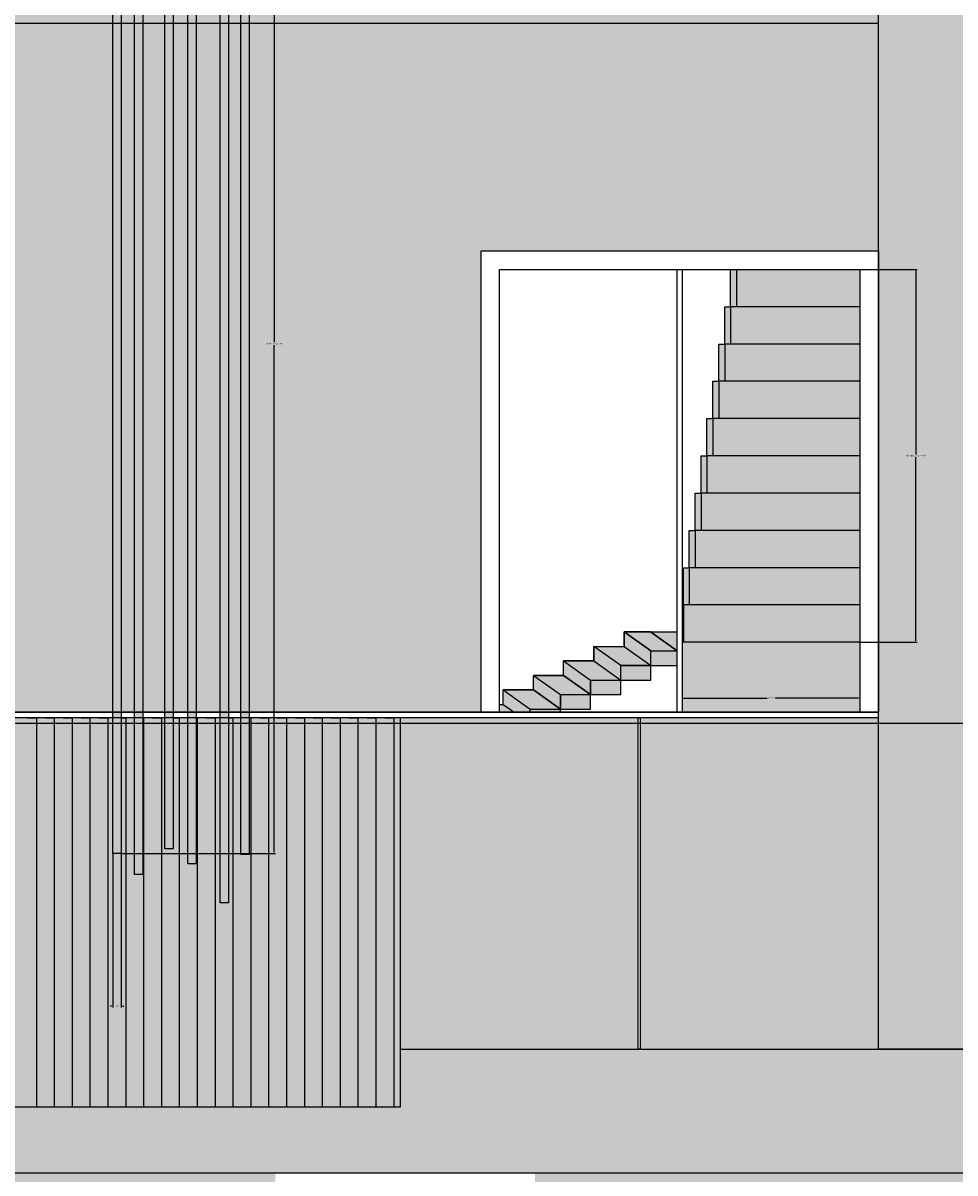
# Model space of a CAD drawing. Units: feet. Extents: x 2193 to 3502, y 890 to 1601.
# Tile 5 of 17: x 2587 to 2710, y 1073 to 1225. Entities that reach past the tile are written whole.
import ezdxf

# ---------------------------------------------------------------- set-up
doc = ezdxf.new("R2010")
doc.units = ezdxf.units.FT
for name, color, linetype, lineweight in [('A-ANNO-DIMS', 2, 'Continuous', 18), ('A-ELEV', 7, 'Continuous', 25), ('A-ELEV-PATT', 8, 'Continuous', 13)]:
    doc.layers.add(name, color=color, linetype=linetype, lineweight=lineweight)
doc.styles.get("Standard").update_dxf_attribs({"font": 'arial.ttf'})
doc.dimstyles.get("Standard").update_dxf_attribs({"dimtxt": 0.18, "dimasz": 0.18, "dimexe": 0.18, "dimexo": 0.0625, "dimgap": 0.09, "dimtad": 0, "dimtih": 1, "dimtoh": 1, "dimdec": 0, "dimzin": 0, "dimdsep": 46, "dimlunit": 3, "dimtxsty": 'Standard', "dimcen": 0.09, "dimadec": 0, "dimazin": 0, "dimtfac": 1, "dimtdec": 0, "dimtofl": 0, "dimtmove": 0, "dimatfit": 3, "dimfxl": 1, "dimtolj": 1, "dimtzin": 0, "dimarcsym": 0})

# ---------------------------------------------------------------- blocks, each defined once
blk = doc.blocks.new('STAIR-RAIL-A')
for p, q in [((6.38, 44.29), (6.38, 49.22)), ((5.61, 39.37), (5.61, 44.29)), ((5.61, 44.29), (6.38, 44.29)), ((23.45, 44.29), (6.38, 44.29)), ((6.38, 44.29), (6.38, 39.37)), ((4.83, 34.45), (4.83, 39.37)), ((4.83, 39.37), (5.61, 39.37)), ((23.45, 39.37), (5.61, 39.37)), ((5.61, 39.37), (5.61, 34.45)), ((4.05, 29.53), (4.05, 34.45)), ((4.05, 34.45), (4.83, 34.45)), ((23.45, 34.45), (4.83, 34.45)), ((4.83, 34.45), (4.83, 29.53)), ((3.27, 24.61), (3.27, 29.53)), ((3.27, 29.53), (4.05, 29.53)), ((23.45, 29.53), (4.05, 29.53)), ((4.05, 29.53), (4.05, 24.61)), ((2.49, 19.69), (2.49, 24.61)), ((2.49, 24.61), (3.27, 24.61)), ((23.45, 24.61), (3.27, 24.61)), ((3.27, 24.61), (3.27, 19.69)), ((1.71, 14.77), (1.71, 19.69)), ((1.71, 19.69), (2.49, 19.69)), ((23.45, 19.69), (2.49, 19.69)), ((2.49, 19.69), (2.49, 14.77)), ((0.93, 9.84), (0.93, 14.77)), ((0.93, 14.77), (1.71, 14.77)), ((23.45, 14.77), (1.71, 14.77)), ((1.71, 14.77), (1.71, 9.84)), ((0.16, 4.92), (0.16, 9.84)), ((0.16, 9.84), (0.93, 9.84)), ((23.45, 9.84), (0.93, 9.84)), ((0.93, 9.84), (0.93, 4.92)), ((23.45, 4.92), (0, 4.92)), ((23.45, 4.92), (0, 4.92)), ((0.16, 4.92), (0.16, 0)), ((23.45, 0), (0, 0)), ((23.45, 0), (0, 0))]:
    blk.add_line(p, q)
for points in [[(23.45, 44.29), (6.38, 44.29), (6.38, 49.22)], [(23.45, 39.37), (5.61, 39.37), (5.61, 44.29), (6.38, 44.29), (6.38, 39.37)], [(23.45, 34.45), (4.83, 34.45), (4.83, 39.37), (5.61, 39.37), (5.61, 34.45)], [(23.45, 29.53), (4.05, 29.53), (4.05, 34.45), (4.83, 34.45), (4.83, 29.53)], [(23.45, 24.61), (3.27, 24.61), (3.27, 29.53), (4.05, 29.53), (4.05, 24.61)], [(23.45, 19.69), (2.49, 19.69), (2.49, 24.61), (3.27, 24.61), (3.27, 19.69)], [(23.45, 14.77), (1.71, 14.77), (1.71, 19.69), (2.49, 19.69), (2.49, 14.77)], [(23.45, 9.84), (0.93, 9.84), (0.93, 14.77), (1.71, 14.77), (1.71, 9.84)], [(0.16, 0), (0.16, 4.92), (0.16, 9.84), (0.93, 9.84), (0.93, 4.92)]]:
    blk.add_lwpolyline(points)
blk = doc.blocks.new('METAL-FIN')
blk.add_lwpolyline([(0, 134.59), (1.1, 134.59), (1.1, 0), (0, 0)], close=True)
blk.add_lwpolyline([(0, 134.59), (1.1, 134.59), (1.1, 0), (0, 0)], close=True)
blk = doc.blocks.new('*D5')
at = {"layer": 'A-ANNO-DIMS', "color": 0, "lineweight": -2, "transparency": 16777216}
for p, q in [((2599.75, 1249.83), (2620.06, 1249.83)), ((2619.88, 1249.65), (2619.88, 1182.71)), ((2619.88, 1115.41), (2619.88, 1182.35)), ((2599.75, 1115.23), (2620.06, 1115.23))]:
    blk.add_line(p, q, dxfattribs=at)
at = {"layer": 'A-ANNO-DIMS', "color": 0, "transparency": 16777216}
for points in [[(2619.85, 1249.65), (2619.91, 1249.65), (2619.88, 1249.83)], [(2619.85, 1115.41), (2619.91, 1115.41), (2619.88, 1115.23)]]:
    blk.add_solid(points, dxfattribs=at)
at = {"layer": 'Defpoints', "color": 0, "transparency": 16777216}
for p in [(2599.69, 1249.83), (2619.88, 1249.83), (2599.69, 1115.23)]:
    blk.add_point(p, dxfattribs=at)
at = {"layer": 'A-ANNO-DIMS', "color": 0, "transparency": 16777216, "insert": (2619.88, 1182.53), "char_height": 0.18, "attachment_point": 5}
blk.add_mtext('\\A1;METAL FIN 135 TYP.', dxfattribs=at)
blk = doc.blocks.new('*D6')
at = {"layer": 'A-ANNO-DIMS', "color": 0, "lineweight": -2, "transparency": 16777216}
for p, q in [((2598.59, 1115.17), (2598.59, 1094.86)), ((2599.69, 1115.17), (2599.69, 1094.86)), ((2598.41, 1095.04), (2598.23, 1095.04)), ((2599.87, 1095.04), (2600.05, 1095.04))]:
    blk.add_line(p, q, dxfattribs=at)
at = {"layer": 'A-ANNO-DIMS', "color": 0, "transparency": 16777216}
for points in [[(2598.41, 1095.07), (2598.41, 1095.01), (2598.59, 1095.04)], [(2599.87, 1095.07), (2599.87, 1095.01), (2599.69, 1095.04)]]:
    blk.add_solid(points, dxfattribs=at)
at = {"layer": 'Defpoints', "color": 0, "transparency": 16777216}
for p in [(2598.59, 1115.23), (2599.69, 1115.23), (2599.69, 1095.04)]:
    blk.add_point(p, dxfattribs=at)
at = {"layer": 'A-ANNO-DIMS', "color": 0, "transparency": 16777216, "insert": (2599.14, 1095.04), "char_height": 0.18, "attachment_point": 5}
blk.add_mtext('\\A1;1 TYP.', dxfattribs=at)
blk = doc.blocks.new('*D7')
at = {"layer": 'A-ANNO-DIMS', "color": 0, "lineweight": -2, "transparency": 16777216}
for p, q in [((2697.25, 1192.33), (2704.75, 1192.33)), ((2704.57, 1192.15), (2704.57, 1167.9)), ((2704.57, 1143.29), (2704.57, 1167.54)), ((2697.25, 1143.11), (2704.75, 1143.11))]:
    blk.add_line(p, q, dxfattribs=at)
at = {"layer": 'A-ANNO-DIMS', "color": 0, "transparency": 16777216}
for points in [[(2704.54, 1192.15), (2704.6, 1192.15), (2704.57, 1192.33)], [(2704.54, 1143.29), (2704.6, 1143.29), (2704.57, 1143.11)]]:
    blk.add_solid(points, dxfattribs=at)
at = {"layer": 'Defpoints', "color": 0, "transparency": 16777216}
for p in [(2697.19, 1192.33), (2704.57, 1192.33), (2697.19, 1143.11)]:
    blk.add_point(p, dxfattribs=at)
at = {"layer": 'A-ANNO-DIMS', "color": 0, "transparency": 16777216, "insert": (2704.57, 1167.72), "char_height": 0.18, "attachment_point": 5}
blk.add_mtext('\\A1;STAIR RAILING A 49 TYP.', dxfattribs=at)
blk = doc.blocks.new('*D8')
at = {"layer": 'A-ANNO-DIMS', "color": 0, "lineweight": -2, "transparency": 16777216}
for p, q in [((2673.73, 1143.05), (2673.73, 1135.55)), ((2697.19, 1143.05), (2697.19, 1135.55)), ((2673.91, 1135.73), (2684.93, 1135.73)), ((2697.01, 1135.73), (2685.99, 1135.73))]:
    blk.add_line(p, q, dxfattribs=at)
at = {"layer": 'A-ANNO-DIMS', "color": 0, "transparency": 16777216}
for points in [[(2673.91, 1135.76), (2673.91, 1135.7), (2673.73, 1135.73)], [(2697.01, 1135.76), (2697.01, 1135.7), (2697.19, 1135.73)]]:
    blk.add_solid(points, dxfattribs=at)
at = {"layer": 'Defpoints', "color": 0, "transparency": 16777216}
for p in [(2673.73, 1143.11), (2697.19, 1143.11), (2697.19, 1135.73)]:
    blk.add_point(p, dxfattribs=at)
at = {"layer": 'A-ANNO-DIMS', "color": 0, "transparency": 16777216, "insert": (2685.46, 1135.73), "char_height": 0.18, "attachment_point": 5}
blk.add_mtext('\\A1;23 TYP.', dxfattribs=at)
blk = doc.blocks.new('*D19')
at = {"layer": 'A-ANNO-DIMS', "color": 0, "lineweight": -2, "transparency": 16777216}
for p, q in [((2934.31, 1073.03), (2193.56, 1073.03)), ((2193.74, 1072.85), (2193.74, 1012.11)), ((2193.74, 951), (2193.74, 1011.75)), ((2934.31, 950.82), (2193.56, 950.82))]:
    blk.add_line(p, q, dxfattribs=at)
at = {"layer": 'A-ANNO-DIMS', "color": 0, "transparency": 16777216}
for points in [[(2193.71, 1072.85), (2193.77, 1072.85), (2193.74, 1073.03)], [(2193.71, 951), (2193.77, 951), (2193.74, 950.82)]]:
    blk.add_solid(points, dxfattribs=at)
at = {"layer": 'Defpoints', "color": 0, "transparency": 16777216}
for p in [(2193.74, 1073.03), (2934.37, 1073.03), (2934.37, 950.82)]:
    blk.add_point(p, dxfattribs=at)
at = {"layer": 'A-ANNO-DIMS', "color": 0, "transparency": 16777216, "insert": (2193.74, 1011.93), "char_height": 0.18, "attachment_point": 5}
blk.add_mtext('\\A1;122.2', dxfattribs=at)
blk = doc.blocks.new('*D20')
at = {"layer": 'A-ANNO-DIMS', "color": 0, "lineweight": -2, "transparency": 16777216}
for p, q in [((2933.15, 1408.48), (2193.56, 1408.48)), ((2193.74, 1408.3), (2193.74, 1240.94)), ((2193.74, 1073.21), (2193.74, 1240.57)), ((2934.31, 1073.03), (2193.56, 1073.03))]:
    blk.add_line(p, q, dxfattribs=at)
at = {"layer": 'A-ANNO-DIMS', "color": 0, "transparency": 16777216}
for points in [[(2193.71, 1408.3), (2193.77, 1408.3), (2193.74, 1408.48)], [(2193.71, 1073.21), (2193.77, 1073.21), (2193.74, 1073.03)]]:
    blk.add_solid(points, dxfattribs=at)
at = {"layer": 'Defpoints', "color": 0, "transparency": 16777216}
for p in [(2193.74, 1408.48), (2933.21, 1408.48), (2934.37, 1073.03)]:
    blk.add_point(p, dxfattribs=at)
at = {"layer": 'A-ANNO-DIMS', "color": 0, "transparency": 16777216, "insert": (2193.74, 1240.76), "char_height": 0.18, "attachment_point": 5}
blk.add_mtext('\\A1;335.45', dxfattribs=at)
blk = doc.blocks.new('*D26')
at = {"layer": 'A-ANNO-DIMS', "color": 0, "lineweight": -2, "transparency": 16777216}
for p, q in [((2255.16, 950.89), (2255.16, 1601.47)), ((2255.34, 1601.29), (2507.42, 1601.29)), ((2760.29, 1601.29), (2508.21, 1601.29)), ((2760.47, 1541.11), (2760.47, 1601.47))]:
    blk.add_line(p, q, dxfattribs=at)
at = {"layer": 'A-ANNO-DIMS', "color": 0, "transparency": 16777216}
for points in [[(2255.34, 1601.32), (2255.34, 1601.26), (2255.16, 1601.29)], [(2760.29, 1601.32), (2760.29, 1601.26), (2760.47, 1601.29)]]:
    blk.add_solid(points, dxfattribs=at)
at = {"layer": 'Defpoints', "color": 0, "transparency": 16777216}
for p in [(2760.47, 1601.29), (2760.47, 1541.04), (2255.16, 950.82)]:
    blk.add_point(p, dxfattribs=at)
at = {"layer": 'A-ANNO-DIMS', "color": 0, "transparency": 16777216, "insert": (2507.82, 1601.29), "char_height": 0.18, "attachment_point": 5}
blk.add_mtext('\\A1;505.3', dxfattribs=at)
blk = doc.blocks.new('*D35')
at = {"layer": 'A-ANNO-DIMS', "color": 0, "lineweight": -2, "transparency": 16777216}
for p, q in [((2980.65, 1132.39), (2193.56, 1132.39)), ((2193.74, 1132.21), (2193.74, 1102.89)), ((2193.74, 1073.21), (2193.74, 1102.53)), ((2934.31, 1073.03), (2193.56, 1073.03))]:
    blk.add_line(p, q, dxfattribs=at)
at = {"layer": 'A-ANNO-DIMS', "color": 0, "transparency": 16777216}
for points in [[(2193.71, 1132.21), (2193.77, 1132.21), (2193.74, 1132.39)], [(2193.71, 1073.21), (2193.77, 1073.21), (2193.74, 1073.03)]]:
    blk.add_solid(points, dxfattribs=at)
at = {"layer": 'Defpoints', "color": 0, "transparency": 16777216}
for p in [(2193.74, 1132.39), (2980.72, 1132.39), (2934.37, 1073.03)]:
    blk.add_point(p, dxfattribs=at)
at = {"layer": 'A-ANNO-DIMS', "color": 0, "transparency": 16777216, "insert": (2193.74, 1102.71), "char_height": 0.18, "attachment_point": 5}
blk.add_mtext('\\A1;59.36', dxfattribs=at)
blk = doc.blocks.new('*D36')
at = {"layer": 'A-ANNO-DIMS', "color": 0, "lineweight": -2, "transparency": 16777216}
for p, q in [((2974.05, 1268.66), (2193.56, 1268.66)), ((2193.74, 1268.48), (2193.74, 1200.71)), ((2193.74, 1132.57), (2193.74, 1200.34)), ((2980.65, 1132.39), (2193.56, 1132.39))]:
    blk.add_line(p, q, dxfattribs=at)
at = {"layer": 'A-ANNO-DIMS', "color": 0, "transparency": 16777216}
for points in [[(2193.71, 1268.48), (2193.77, 1268.48), (2193.74, 1268.66)], [(2193.71, 1132.57), (2193.77, 1132.57), (2193.74, 1132.39)]]:
    blk.add_solid(points, dxfattribs=at)
at = {"layer": 'Defpoints', "color": 0, "transparency": 16777216}
for p in [(2193.74, 1268.66), (2974.12, 1268.66), (2980.72, 1132.39)]:
    blk.add_point(p, dxfattribs=at)
at = {"layer": 'A-ANNO-DIMS', "color": 0, "transparency": 16777216, "insert": (2193.74, 1200.53), "char_height": 0.18, "attachment_point": 5}
blk.add_mtext('\\A1;136.27', dxfattribs=at)

msp = doc.modelspace()

# ---------------------------------------------------------------- hatches: boundary and pattern name
at = {"layer": 'A-ELEV-PATT'}
h = msp.add_hatch(color=256, dxfattribs=at)
h.dxf.hatch_style = 1
h.paths.add_polyline_path([(2760.4733, 1541.0441), (2699.6322, 1541.0441), (2699.6322, 1512.3957), (2760.4733, 1512.3957)])
h.paths.add_polyline_path([(2760.4733, 1502.0763), (2699.6322, 1502.0763), (2699.6322, 1382.0763), (2760.4733, 1382.0763)])
h.paths.add_polyline_path([(2745.971, 1367.5739), (2699.6322, 1367.5739), (2699.6322, 1089.3627), (2760.4733, 1089.3627), (2760.4733, 1166.2327), (2745.971, 1166.2327)])
h.paths.add_polyline_path([(2754.7661, 1011.1246), (2690.9216, 1011.1246), (2690.9216, 993.3923), (2754.7661, 993.3923)])
h.paths.add_polyline_path([(2689.6008, 1011.1246), (2625.7563, 1011.1246), (2625.7563, 993.3923), (2689.6008, 993.3923)])
h.paths.add_polyline_path([(2599.6883, 1249.8256), (2598.591, 1249.8256), (2598.591, 1233.561), (2599.6883, 1233.561)])
h.paths.add_polyline_path([(2602.5204, 1247.0422), (2601.423, 1247.0422), (2601.423, 1233.561), (2602.5204, 1233.561)])
h.paths.add_polyline_path([(2606.5316, 1250.4403), (2605.4342, 1250.4403), (2605.4342, 1233.561), (2606.5316, 1233.561)])
h.paths.add_polyline_path([(2609.5836, 1248.4363), (2608.4862, 1248.4363), (2608.4862, 1233.561), (2609.5836, 1233.561)])
h.paths.add_polyline_path([(2613.8564, 1243.2956), (2612.759, 1243.2956), (2612.759, 1233.561), (2613.8564, 1233.561)])
h.paths.add_polyline_path([(2616.5596, 1249.6561), (2615.4622, 1249.6561), (2615.4622, 1233.561), (2616.5596, 1233.561)])
h.paths.add_polyline_path([(2599.6883, 1233.561), (2598.591, 1233.561), (2598.591, 1224.865), (2599.6883, 1224.865)])
h.paths.add_polyline_path([(2602.5204, 1233.561), (2601.423, 1233.561), (2601.423, 1224.865), (2602.5204, 1224.865)])
h.paths.add_polyline_path([(2606.5316, 1233.561), (2605.4342, 1233.561), (2605.4342, 1224.865), (2606.5316, 1224.865)])
h.paths.add_polyline_path([(2609.5836, 1233.561), (2608.4862, 1233.561), (2608.4862, 1224.865), (2609.5836, 1224.865)])
h.paths.add_polyline_path([(2613.8564, 1233.561), (2612.759, 1233.561), (2612.759, 1224.865), (2613.8564, 1224.865)])
h.paths.add_polyline_path([(2616.5596, 1233.561), (2615.4622, 1233.561), (2615.4622, 1224.865), (2616.5596, 1224.865)])
h.paths.add_polyline_path([(2599.6883, 1224.865), (2598.591, 1224.865), (2598.591, 1115.2331), (2599.6883, 1115.2331)])
h.paths.add_polyline_path([(2602.5204, 1224.865), (2601.423, 1224.865), (2601.423, 1112.4498), (2602.5204, 1112.4498)])
h.paths.add_polyline_path([(2606.5316, 1224.865), (2605.4342, 1224.865), (2605.4342, 1115.8479), (2606.5316, 1115.8479)])
h.paths.add_polyline_path([(2609.5836, 1224.865), (2608.4862, 1224.865), (2608.4862, 1113.8439), (2609.5836, 1113.8439)])
h.paths.add_polyline_path([(2616.5596, 1224.865), (2615.4622, 1224.865), (2615.4622, 1115.0637), (2616.5596, 1115.0637)])
h.paths.add_polyline_path([(2613.8564, 1224.865), (2612.759, 1224.865), (2612.759, 1108.7032), (2613.8564, 1108.7032)])
h = msp.add_hatch(color=256, dxfattribs=at)
h.dxf.hatch_style = 1
h.paths.add_polyline_path([(2390.8933, 1367.5739), (2294.8992, 1367.5739), (2294.8992, 1329.5765), (2390.8933, 1329.5765)])
h.paths.add_polyline_path([(2489.6169, 1055.3069), (2585.8844, 1055.3069), (2585.8844, 1032.1935), (2620.0491, 1032.1935), (2620.0491, 1073.031), (2452.7821, 1073.031), (2452.7821, 1032.1935), (2489.6169, 1032.1935)])
h.paths.add_polyline_path([(2754.7661, 1073.031), (2654.2841, 1073.031), (2654.2841, 1047.0961), (2754.7661, 1047.0961)])
h.paths.add_polyline_path([(2643.9681, 1484.1152), (2699.5726, 1484.1152), (2699.5726, 1502.0763), (2602.8648, 1502.0763), (2602.8648, 1408.4814), (2643.9681, 1408.4814)])
h.paths.add_polyline_path([(2699.6322, 1367.5739), (2646.2844, 1367.5739), (2646.2844, 1268.6599), (2647.1841, 1268.6599), (2647.1841, 1329.5765), (2699.6322, 1329.5765)])
h.paths.add_polyline_path([(2699.6322, 1224.865), (2616.5596, 1224.865), (2616.5596, 1133.8558), (2647.1841, 1133.8558), (2647.1841, 1194.7724), (2699.6322, 1194.7724)])
h = msp.add_hatch(color=256, dxfattribs=at)
h.dxf.hatch_style = 1
h.paths.add_polyline_path([(2576.3428, 1407.7384), (2536.5416, 1407.7384), (2536.5416, 1406.15), (2536.5416, 1382.0763), (2576.3428, 1382.0763)])
h.paths.add_polyline_path([(2627.3548, 1407.7384), (2576.5924, 1407.7384), (2576.5924, 1382.0763), (2627.3548, 1382.0763)])
h.paths.add_polyline_path([(2667.9236, 1407.7384), (2627.6045, 1407.7384), (2627.6045, 1382.0763), (2667.9236, 1382.0763)])
h.paths.add_polyline_path([(2699.6322, 1407.7384), (2668.1733, 1407.7384), (2668.1733, 1382.0763), (2699.6322, 1382.0763)])
h.paths.add_polyline_path([(2497.5717, 1323.2248), (2470.7305, 1323.2248), (2470.7305, 1271.105), (2497.5717, 1271.105)])
h.paths.add_polyline_path([(2577.3219, 1323.2248), (2500.599, 1323.2248), (2500.599, 1271.105), (2577.3219, 1271.105)])
h.paths.add_polyline_path([(2388.4482, 1327.1314), (2343.4244, 1327.1314), (2343.4244, 1268.6599), (2388.4482, 1268.6599)])
h.paths.add_polyline_path([(2342.3682, 1327.1314), (2297.3443, 1327.1314), (2297.3443, 1268.6599), (2342.3682, 1268.6599)])
h.paths.add_polyline_path([(2335.8632, 1214.8367), (2301.4984, 1214.8367), (2301.4984, 1133.1367), (2335.8632, 1133.1367)])
h.paths.add_polyline_path([(2371.1246, 1214.8367), (2337.2323, 1214.8367), (2337.2323, 1133.1367), (2371.1246, 1133.1367)])
h.paths.add_polyline_path([(2390.8933, 1214.8367), (2372.4936, 1214.8367), (2372.4936, 1133.1367), (2390.8933, 1133.1367)])
h.paths.add_polyline_path([(2577.3219, 1188.4208), (2500.599, 1188.4208), (2500.599, 1136.3009), (2577.3219, 1136.3009)])
h.paths.add_polyline_path([(2497.5717, 1188.4208), (2470.7305, 1188.4208), (2470.7305, 1136.3009), (2497.5717, 1136.3009)])
h.paths.add_polyline_path([(2381.4675, 1132.3937), (2301.4984, 1132.3937), (2301.4984, 1085.6301), (2381.4675, 1085.6301)])
h.paths.add_polyline_path([(2461.6863, 1132.3937), (2381.7172, 1132.3937), (2381.7172, 1085.6301), (2461.6863, 1085.6301)])
h.paths.add_polyline_path([(2494.0463, 1133.1128), (2468.2854, 1133.1128), (2468.2854, 1089.3627), (2494.0463, 1089.3627)])
h.paths.add_polyline_path([(2517.7591, 1133.1128), (2494.296, 1133.1128), (2494.296, 1089.3627), (2517.7591, 1089.3627)])
h.paths.add_polyline_path([(2667.9236, 1133.1128), (2636.5184, 1133.1128), (2636.5184, 1089.3627), (2667.9236, 1089.3627)])
h.paths.add_polyline_path([(2699.6322, 1133.1128), (2668.1733, 1133.1128), (2668.1733, 1089.3627), (2699.6322, 1089.3627)])
h.paths.add_polyline_path([(2651.839, 1070.5859), (2638.7977, 1070.5859), (2638.7977, 1047.0961), (2651.839, 1047.0961)])
h.paths.add_polyline_path([(2637.6317, 1070.5859), (2625.7563, 1070.5859), (2625.7563, 1047.0961), (2637.6317, 1047.0961)])
h.paths.add_polyline_path([(2583.4393, 1052.8618), (2515.9216, 1052.8618), (2515.9216, 1032.1935), (2583.4393, 1032.1935)])
h.paths.add_polyline_path([(2514.4293, 1052.8618), (2492.062, 1052.8618), (2492.062, 1032.1935), (2514.4293, 1032.1935)])
h.paths.add_polyline_path([(2388.4482, 1038.8658), (2348.7682, 1038.8658), (2348.7682, 988.9597), (2388.4482, 988.9597)])
h.paths.add_polyline_path([(2346.3231, 1038.8658), (2309.0883, 1038.8658), (2309.0883, 988.9597), (2346.3231, 988.9597)])
h.paths.add_polyline_path([(2667.9236, 1267.9169), (2636.5184, 1267.9169), (2636.5184, 1241.1967), (2667.9236, 1241.1967)])
h.paths.add_polyline_path([(2699.6322, 1267.9169), (2668.1733, 1267.9169), (2668.1733, 1241.1967), (2699.6322, 1241.1967)])
h.paths.add_polyline_path([(2517.7591, 1267.9169), (2494.296, 1267.9169), (2494.296, 1241.1967), (2517.7591, 1241.1967)])
h.paths.add_polyline_path([(2494.0463, 1267.9169), (2468.2854, 1267.9169), (2468.2854, 1266.7092), (2468.2854, 1241.1967), (2494.0463, 1241.1967)])
h = msp.add_hatch(color=256, dxfattribs=at)
h.dxf.hatch_style = 1
h.paths.add_polyline_path([(2294.8992, 1367.5739), (2275.0482, 1367.5739), (2275.0482, 1382.0763), (2536.5416, 1382.0763), (2536.5416, 1406.15), (2256.3232, 1406.15), (2256.3232, 1089.3627), (2255.1574, 1089.3627), (2255.1574, 1073.031), (2294.8992, 1073.031)])
h.paths.add_polyline_path([(2517.7591, 1241.1967), (2468.2854, 1241.1967), (2468.2854, 1224.865), (2598.591, 1224.865), (2598.591, 1233.561), (2517.7591, 1233.561)])
h.paths.add_polyline_path([(2699.6322, 1241.1967), (2636.5184, 1241.1967), (2636.5184, 1233.561), (2616.5596, 1233.561), (2616.5596, 1224.865), (2699.6322, 1224.865)])
h.paths.add_polyline_path([(2615.4622, 1233.561), (2613.8564, 1233.561), (2613.8564, 1224.865), (2615.4622, 1224.865)])
h.paths.add_polyline_path([(2612.759, 1233.561), (2609.5836, 1233.561), (2609.5836, 1224.865), (2612.759, 1224.865)])
h.paths.add_polyline_path([(2608.4862, 1233.561), (2606.5316, 1233.561), (2606.5316, 1224.865), (2608.4862, 1224.865)])
h.paths.add_polyline_path([(2605.4342, 1233.561), (2602.5204, 1233.561), (2602.5204, 1224.865), (2605.4342, 1224.865)])
h.paths.add_polyline_path([(2601.423, 1233.561), (2599.6883, 1233.561), (2599.6883, 1224.865), (2601.423, 1224.865)])
h.paths.add_polyline_path([(2517.7591, 1089.3627), (2468.2854, 1089.3627), (2468.2854, 1079.031), (2294.8992, 1079.031), (2294.8992, 1073.031), (2390.8933, 1073.031), (2452.7821, 1073.031), (2760.4733, 1073.031), (2760.4733, 1089.3627), (2699.6322, 1089.3627), (2636.5184, 1089.3627), (2636.5184, 1081.7269), (2517.7591, 1081.7269)])
h = msp.add_hatch(color=256, dxfattribs=at)
h.dxf.hatch_style = 1
h.paths.add_polyline_path([(2452.7821, 1355.2199), (2622.9814, 1355.2199), (2622.9814, 1268.6599), (2646.2844, 1268.6599), (2646.2844, 1367.5739), (2390.8933, 1367.5739), (2390.8933, 1268.6599), (2452.7821, 1268.6599)])
h.paths.add_polyline_path([(2452.7821, 1016.4), (2431.9134, 1016.4), (2431.9134, 1032.1935), (2452.7821, 1032.1935), (2452.7821, 1073.031), (2390.8933, 1073.031), (2390.8933, 956.8829), (2452.7821, 956.8829)])
h.paths.add_polyline_path([(2452.7821, 1241.1967), (2390.8933, 1241.1967), (2390.8933, 1133.1367), (2452.7821, 1133.1367)])
h.paths.add_polyline_path([(2636.5184, 1267.9169), (2517.7591, 1267.9169), (2517.7591, 1233.561), (2598.591, 1233.561), (2598.591, 1249.8256), (2599.6883, 1249.8256), (2599.6883, 1233.561), (2601.423, 1233.561), (2601.423, 1247.0422), (2602.5204, 1247.0422), (2602.5204, 1233.561), (2605.4342, 1233.561), (2605.4342, 1250.4403), (2606.5316, 1250.4403), (2606.5316, 1233.561), (2608.4862, 1233.561), (2608.4862, 1248.4363), (2609.5836, 1248.4363), (2609.5836, 1233.561), (2612.759, 1233.561), (2612.759, 1243.2956), (2613.8564, 1243.2956), (2613.8564, 1233.561), (2615.4622, 1233.561), (2615.4622, 1249.6561), (2616.5596, 1249.6561), (2616.5596, 1233.561), (2636.5184, 1233.561)])
h.paths.add_polyline_path([(2601.423, 1133.1128), (2599.6883, 1133.1128), (2599.6883, 1115.2331), (2598.591, 1115.2331), (2598.591, 1133.1128), (2517.7591, 1133.1128), (2517.7591, 1081.7269), (2636.5184, 1081.7269), (2636.5184, 1133.1128), (2616.5596, 1133.1128), (2616.5596, 1115.0637), (2615.4622, 1115.0637), (2615.4622, 1133.1128), (2613.8564, 1133.1128), (2613.8564, 1108.7032), (2612.759, 1108.7032), (2612.759, 1133.1128), (2609.5836, 1133.1128), (2609.5836, 1113.8439), (2608.4862, 1113.8439), (2608.4862, 1133.1128), (2606.5316, 1133.1128), (2606.5316, 1115.8479), (2605.4342, 1115.8479), (2605.4342, 1133.1128), (2602.5204, 1133.1128), (2602.5204, 1112.4498), (2601.423, 1112.4498)])
h = msp.add_hatch(color=256, dxfattribs=at)
h.dxf.hatch_style = 1
h.paths.add_polyline_path([(2622.9814, 1355.2199), (2452.7821, 1355.2199), (2452.7821, 1268.6599), (2468.2854, 1268.6599), (2468.2854, 1325.6699), (2579.767, 1325.6699), (2579.767, 1268.6599), (2622.9814, 1268.6599)])
h.paths.add_polyline_path([(2598.591, 1224.865), (2468.2854, 1224.865), (2468.2854, 1190.8659), (2579.767, 1190.8659), (2579.767, 1133.8558), (2598.591, 1133.8558)])
h.paths.add_polyline_path([(2390.8933, 1241.1967), (2301.4984, 1241.1967), (2301.4984, 1224.865), (2390.8933, 1224.865)])
h.paths.add_polyline_path([(3070.1101, 1073.031), (2940.0814, 1073.031), (2940.0814, 956.5285), (2940.6598, 956.8829), (3070.1101, 956.8829), (3070.1101, 986.5146), (2985.8599, 986.5146), (2985.8599, 1041.3109), (3070.1101, 1041.3109)])
h = msp.add_hatch(color=256, dxfattribs=at)
h.dxf.hatch_style = 1
h.paths.add_polyline_path([(2697.1871, 1322.2098), (2680.1178, 1322.2098), (2680.1178, 1317.2882), (2697.1871, 1317.2882)])
h.paths.add_polyline_path([(2697.1871, 1327.1314), (2680.8966, 1327.1314), (2680.8966, 1322.2098), (2697.1871, 1322.2098)])
h.paths.add_polyline_path([(2697.1871, 1317.2882), (2679.3391, 1317.2882), (2679.3391, 1312.3666), (2697.1871, 1312.3666)])
h.paths.add_polyline_path([(2697.1871, 1312.3666), (2678.5604, 1312.3666), (2678.5604, 1307.445), (2697.1871, 1307.445)])
h.paths.add_polyline_path([(2697.1871, 1307.445), (2677.7817, 1307.445), (2677.7817, 1302.5234), (2697.1871, 1302.5234)])
h.paths.add_polyline_path([(2697.1871, 1302.5234), (2677.0029, 1302.5234), (2677.0029, 1297.6018), (2697.1871, 1297.6018)])
h.paths.add_polyline_path([(2697.1871, 1297.6018), (2676.2242, 1297.6018), (2676.2242, 1292.6802), (2697.1871, 1292.6802)])
h.paths.add_polyline_path([(2697.1871, 1292.6802), (2675.4455, 1292.6802), (2675.4455, 1287.7586), (2697.1871, 1287.7586)])
h.paths.add_polyline_path([(2697.1871, 1287.7586), (2674.6667, 1287.7586), (2673.888, 1287.7586), (2673.888, 1282.8371), (2673.888, 1277.9155), (2673.7332, 1268.6599), (2697.1871, 1268.6599)])
h.paths.add_polyline_path([(2662.0707, 1275.4405), (2658.0881, 1275.4405), (2661.6386, 1272.9217), (2665.6211, 1272.9217)])
h.paths.add_polyline_path([(2666.0533, 1279.2756), (2666.0533, 1277.358), (2669.6037, 1274.8393), (2669.6037, 1276.7569)])
h.paths.add_polyline_path([(2669.5328, 1279.2756), (2666.0533, 1279.2756), (2669.6037, 1276.7569), (2673.0832, 1276.7569)])
h.paths.add_polyline_path([(2673.0832, 1279.2756), (2669.5328, 1279.2756), (2673.0832, 1276.7569)], flags=17)
h.paths.add_polyline_path([(2673.0832, 1276.7569), (2669.6037, 1276.7569), (2669.6037, 1274.8393), (2673.0832, 1274.8393)])
h.paths.add_polyline_path([(2669.6037, 1274.8393), (2665.6211, 1274.8393), (2665.6211, 1272.9217), (2669.6037, 1272.9217)])
h.paths.add_polyline_path([(2666.0533, 1277.358), (2662.0707, 1277.358), (2665.6211, 1274.8393), (2669.6037, 1274.8393)])
h.paths.add_polyline_path([(2662.0707, 1277.358), (2662.0707, 1275.4405), (2665.6211, 1272.9217), (2665.6211, 1274.8393)])
h.paths.add_polyline_path([(2665.6211, 1272.9217), (2661.6386, 1272.9217), (2661.6386, 1271.0041), (2665.6211, 1271.0041)])
h.paths.add_polyline_path([(2658.0881, 1275.4405), (2658.0881, 1273.5229), (2661.6386, 1271.0041), (2661.6386, 1272.9217)])
h.paths.add_polyline_path([(2661.6386, 1271.0041), (2657.656, 1271.0041), (2657.656, 1269.0866), (2661.6386, 1269.0866)])
h.paths.add_polyline_path([(2658.0881, 1273.5229), (2654.1056, 1273.5229), (2657.656, 1271.0041), (2661.6386, 1271.0041)])
h.paths.add_polyline_path([(2654.1056, 1273.5229), (2654.1056, 1271.6053), (2657.656, 1269.0866), (2657.656, 1271.0041)])
h.paths.add_polyline_path([(2650.123, 1271.6053), (2650.123, 1269.6877), (2651.5719, 1268.6599), (2653.6734, 1268.6599), (2653.6734, 1269.0866)])
h.paths.add_polyline_path([(2654.1056, 1271.6053), (2650.123, 1271.6053), (2653.6734, 1269.0866), (2657.656, 1269.0866)])
h.paths.add_polyline_path([(2650.123, 1269.6877), (2649.6293, 1269.6877), (2649.6293, 1268.6599), (2651.5719, 1268.6599)])
h.paths.add_polyline_path([(2657.656, 1269.0866), (2653.6734, 1269.0866), (2653.6734, 1268.6599), (2657.656, 1268.6599)])
h.paths.add_polyline_path([(2697.1871, 1192.3273), (2680.8966, 1192.3273), (2680.8966, 1187.4057), (2697.1871, 1187.4057)])
h.paths.add_polyline_path([(2697.1871, 1187.4057), (2680.1178, 1187.4057), (2680.1178, 1182.4841), (2697.1871, 1182.4841)])
h.paths.add_polyline_path([(2697.1871, 1177.5625), (2678.5604, 1177.5625), (2678.5604, 1172.641), (2697.1871, 1172.641)])
h.paths.add_polyline_path([(2697.1871, 1182.4841), (2679.3391, 1182.4841), (2679.3391, 1177.5625), (2697.1871, 1177.5625)])
h.paths.add_polyline_path([(2697.1871, 1172.641), (2677.7817, 1172.641), (2677.7817, 1167.7194), (2697.1871, 1167.7194)])
h.paths.add_polyline_path([(2697.1871, 1167.7194), (2677.0029, 1167.7194), (2677.0029, 1162.7978), (2697.1871, 1162.7978)])
h.paths.add_polyline_path([(2697.1871, 1162.7978), (2676.2242, 1162.7978), (2676.2242, 1157.8762), (2697.1871, 1157.8762)])
h.paths.add_polyline_path([(2697.1871, 1143.1114), (2673.7332, 1143.1114), (2673.7332, 1133.8558), (2697.1871, 1133.8558)])
h.paths.add_polyline_path([(2697.1871, 1148.033), (2673.888, 1148.033), (2673.888, 1143.1114), (2697.1871, 1143.1114)])
h.paths.add_polyline_path([(2697.1871, 1152.9546), (2674.6667, 1152.9546), (2674.6667, 1148.033), (2697.1871, 1148.033)])
h.paths.add_polyline_path([(2697.1871, 1157.8762), (2675.4455, 1157.8762), (2675.4455, 1152.9546), (2697.1871, 1152.9546)])
h.paths.add_polyline_path([(2673.0832, 1141.9528), (2669.6037, 1141.9528), (2669.6037, 1140.0352), (2673.0832, 1140.0352)])
h.paths.add_polyline_path([(2669.5328, 1144.4716), (2666.0533, 1144.4716), (2669.6037, 1141.9528), (2673.0832, 1141.9528)])
h.paths.add_polyline_path([(2673.0832, 1144.4716), (2669.5328, 1144.4716), (2673.0832, 1141.9528)], flags=17)
h.paths.add_polyline_path([(2666.0533, 1142.554), (2662.0707, 1142.554), (2665.6211, 1140.0352), (2669.6037, 1140.0352)])
h.paths.add_polyline_path([(2666.0533, 1144.4716), (2666.0533, 1142.554), (2669.6037, 1140.0352), (2669.6037, 1141.9528)])
h.paths.add_polyline_path([(2669.6037, 1140.0352), (2665.6211, 1140.0352), (2665.6211, 1138.1177), (2669.6037, 1138.1177)])
h.paths.add_polyline_path([(2665.6211, 1140.0352), (2662.0707, 1142.554), (2662.0707, 1140.6364), (2665.6211, 1138.1177)])
h.paths.add_polyline_path([(2653.6734, 1134.2825), (2650.123, 1136.8013), (2650.123, 1134.8837), (2651.5719, 1133.8558), (2653.6734, 1133.8558)])
h.paths.add_polyline_path([(2654.1056, 1136.8013), (2650.123, 1136.8013), (2653.6734, 1134.2825), (2657.656, 1134.2825)])
h.paths.add_polyline_path([(2657.656, 1134.2825), (2653.6734, 1134.2825), (2653.6734, 1133.8558), (2657.656, 1133.8558)])
h.paths.add_polyline_path([(2661.6386, 1136.2001), (2657.656, 1136.2001), (2657.656, 1134.2825), (2661.6386, 1134.2825)])
h.paths.add_polyline_path([(2657.656, 1136.2001), (2654.1056, 1138.7188), (2654.1056, 1136.8013), (2657.656, 1134.2825)])
h.paths.add_polyline_path([(2658.0881, 1138.7188), (2654.1056, 1138.7188), (2657.656, 1136.2001), (2661.6386, 1136.2001)])
h.paths.add_polyline_path([(2658.0881, 1140.6364), (2658.0881, 1138.7188), (2661.6386, 1136.2001), (2661.6386, 1138.1177)])
h.paths.add_polyline_path([(2662.0707, 1140.6364), (2658.0881, 1140.6364), (2661.6386, 1138.1177), (2665.6211, 1138.1177)])
h.paths.add_polyline_path([(2665.6211, 1138.1177), (2661.6386, 1138.1177), (2661.6386, 1136.2001), (2665.6211, 1136.2001)])
h.paths.add_polyline_path([(2650.123, 1134.8837), (2649.6293, 1134.8837), (2649.6293, 1133.8558), (2651.5719, 1133.8558)])
h = msp.add_hatch(color=256, dxfattribs=at)
h.dxf.hatch_style = 1
h.paths.add_polyline_path([(2680.8966, 1327.1314), (2680.1178, 1327.1314), (2680.1178, 1322.2098), (2680.8966, 1322.2098)])
h.paths.add_polyline_path([(2680.1178, 1322.2098), (2679.3391, 1322.2098), (2679.3391, 1317.2882), (2680.1178, 1317.2882)])
h.paths.add_polyline_path([(2679.3391, 1317.2882), (2678.5604, 1317.2882), (2678.5604, 1312.3666), (2679.3391, 1312.3666)])
h.paths.add_polyline_path([(2678.5604, 1312.3666), (2677.7817, 1312.3666), (2677.7817, 1307.445), (2678.5604, 1307.445)])
h.paths.add_polyline_path([(2677.7817, 1307.445), (2677.0029, 1307.445), (2677.0029, 1302.5234), (2677.7817, 1302.5234)])
h.paths.add_polyline_path([(2677.0029, 1302.5234), (2676.2242, 1302.5234), (2676.2242, 1297.6018), (2677.0029, 1297.6018)])
h.paths.add_polyline_path([(2676.2242, 1297.6018), (2675.4455, 1297.6018), (2675.4455, 1292.6802), (2676.2242, 1292.6802)])
h.paths.add_polyline_path([(2675.4455, 1292.6802), (2674.6667, 1292.6802), (2674.6667, 1287.7586), (2675.4455, 1287.7586)])
h.paths.add_polyline_path([(2680.8966, 1192.3273), (2680.1178, 1192.3273), (2680.1178, 1187.4057), (2680.8966, 1187.4057)])
h.paths.add_polyline_path([(2680.1178, 1187.4057), (2679.3391, 1187.4057), (2679.3391, 1182.4841), (2680.1178, 1182.4841)])
h.paths.add_polyline_path([(2679.3391, 1182.4841), (2678.5604, 1182.4841), (2678.5604, 1177.5625), (2679.3391, 1177.5625)])
h.paths.add_polyline_path([(2678.5604, 1177.5625), (2677.7817, 1177.5625), (2677.7817, 1172.641), (2678.5604, 1172.641)])
h.paths.add_polyline_path([(2677.7817, 1172.641), (2677.0029, 1172.641), (2677.0029, 1167.7194), (2677.7817, 1167.7194)])
h = msp.add_hatch(color=256, dxfattribs=at)
h.dxf.hatch_style = 1
h.paths.add_polyline_path([(2601.423, 1224.865), (2599.6883, 1224.865), (2599.6883, 1133.8558), (2601.423, 1133.8558)])
h.paths.add_polyline_path([(2605.4342, 1224.865), (2602.5204, 1224.865), (2602.5204, 1133.8558), (2605.4342, 1133.8558)])
h.paths.add_polyline_path([(2608.4862, 1224.865), (2606.5316, 1224.865), (2606.5316, 1133.8558), (2608.4862, 1133.8558)])
h.paths.add_polyline_path([(2612.759, 1224.865), (2609.5836, 1224.865), (2609.5836, 1133.8558), (2612.759, 1133.8558)])
h.paths.add_polyline_path([(2615.4622, 1224.865), (2613.8564, 1224.865), (2613.8564, 1133.8558), (2615.4622, 1133.8558)])
h = msp.add_hatch(color=256, dxfattribs=at)
h.dxf.hatch_style = 1
h.paths.add_polyline_path([(2677.0029, 1167.7194), (2676.2242, 1167.7194), (2676.2242, 1162.7978), (2677.0029, 1162.7978)])
h = msp.add_hatch(color=256, dxfattribs=at)
h.dxf.hatch_style = 1
h.paths.add_polyline_path([(2674.6667, 1152.9546), (2673.888, 1152.9546), (2673.888, 1148.033), (2674.6667, 1148.033)])
h.paths.add_polyline_path([(2675.4455, 1157.8762), (2674.6667, 1157.8762), (2674.6667, 1152.9546), (2675.4455, 1152.9546)])
h.paths.add_polyline_path([(2676.2242, 1162.7978), (2675.4455, 1162.7978), (2675.4455, 1157.8762), (2676.2242, 1157.8762)])

# ---------------------------------------------------------------- linework, layer by layer
at = {"layer": 'A-ELEV'}
for p, q in [((2468.2854, 1224.865), (2699.6322, 1224.865)), ((2680.8966, 1192.3273), (2680.8966, 1187.4057)), ((2680.8966, 1192.3273), (2680.8966, 1187.4057)), ((2669.6037, 1141.9528), (2666.0533, 1144.4716)), ((2666.0533, 1144.4716), (2669.5328, 1144.4716)), ((2666.0533, 1142.554), (2666.0533, 1144.4716)), ((2669.5328, 1144.4716), (2673.0832, 1141.9528)), ((2669.5328, 1144.4716), (2673.0832, 1144.4716)), ((2662.0707, 1142.554), (2666.0533, 1142.554)), ((2662.0707, 1140.6364), (2662.0707, 1142.554)), ((2662.0707, 1142.554), (2666.0533, 1142.554)), ((2665.6211, 1140.0352), (2662.0707, 1142.554)), ((2666.0533, 1142.554), (2669.6037, 1140.0352)), ((2669.6037, 1140.0352), (2669.6037, 1141.9528)), ((2669.6037, 1141.9528), (2673.0832, 1141.9528)), ((2658.0881, 1138.7188), (2658.0881, 1140.6364)), ((2658.0881, 1138.7188), (2658.0881, 1140.6364)), ((2658.0881, 1140.6364), (2662.0707, 1140.6364)), ((2658.0881, 1140.6364), (2661.6386, 1138.1177)), ((2662.0707, 1140.6364), (2665.6211, 1138.1177)), ((2665.6211, 1138.1177), (2665.6211, 1140.0352)), ((2665.6211, 1140.0352), (2669.6037, 1140.0352)), ((2669.6037, 1140.0352), (2673.0832, 1140.0352)), ((2669.6037, 1138.1177), (2669.6037, 1140.0352)), ((2654.1056, 1136.8013), (2654.1056, 1138.7188)), ((2654.1056, 1136.8013), (2654.1056, 1138.7188)), ((2654.1056, 1138.7188), (2658.0881, 1138.7188)), ((2654.1056, 1138.7188), (2657.656, 1136.2001)), ((2658.0881, 1138.7188), (2661.6386, 1136.2001)), ((2661.6386, 1136.2001), (2661.6386, 1138.1177)), ((2661.6386, 1138.1177), (2665.6211, 1138.1177)), ((2665.6211, 1136.2001), (2665.6211, 1138.1177)), ((2665.6211, 1138.1177), (2669.6037, 1138.1177)), ((2650.123, 1134.8837), (2650.123, 1136.8013)), ((2650.123, 1134.8837), (2650.123, 1136.8013)), ((2650.123, 1136.8013), (2654.1056, 1136.8013)), ((2650.123, 1136.8013), (2653.6734, 1134.2825)), ((2654.1056, 1136.8013), (2657.656, 1134.2825)), ((2657.656, 1134.2825), (2657.656, 1136.2001)), ((2657.656, 1136.2001), (2661.6386, 1136.2001)), ((2661.6386, 1134.2825), (2661.6386, 1136.2001)), ((2661.6386, 1136.2001), (2665.6211, 1136.2001)), ((2649.6293, 1134.8837), (2650.123, 1134.8837)), ((2650.123, 1134.8837), (2651.5719, 1133.8558)), ((2653.6734, 1133.8558), (2653.6734, 1134.2825)), ((2653.6734, 1134.2825), (2657.656, 1134.2825)), ((2657.656, 1133.8558), (2657.656, 1134.2825)), ((2657.656, 1134.2825), (2661.6386, 1134.2825)), ((2653.6734, 1133.8558), (2653.6734, 1133.8558)), ((2636.5184, 1089.3627), (2760.4733, 1089.3627)), ((2636.5184, 1089.3627), (2760.4733, 1089.3627))]:
    msp.add_line(p, q, dxfattribs=at)
for points in [[(2760.4733, 1415.3157), (2760.4733, 1089.3627), (2699.6322, 1089.3627), (2699.6322, 1367.5739)], [(2760.4733, 1415.3157), (2760.4733, 1089.3627), (2699.6322, 1089.3627), (2699.6322, 1367.5739)], [(2649.6293, 1133.8558), (2649.6293, 1192.3273), (2697.1871, 1192.3273), (2697.1871, 1133.8558)], [(2649.6293, 1133.8558), (2649.6293, 1192.3273), (2697.1871, 1192.3273), (2697.1871, 1133.8558)], [(2669.5328, 1144.4716), (2666.0533, 1144.4716), (2666.0533, 1142.554), (2669.6037, 1140.0352), (2669.6037, 1141.9528)], [(2666.0533, 1144.4716), (2669.6037, 1141.9528), (2673.0832, 1141.9528), (2669.5328, 1144.4716), (2673.0832, 1144.4716)], [(2669.6037, 1140.0352), (2665.6211, 1140.0352), (2662.0707, 1142.554), (2662.0707, 1140.6364), (2665.6211, 1138.1177), (2665.6211, 1140.0352)], [(2662.0707, 1140.6364), (2658.0881, 1140.6364), (2661.6386, 1138.1177), (2665.6211, 1138.1177)], [(2657.656, 1133.8558), (2657.656, 1134.2825), (2661.6386, 1134.2825), (2661.6386, 1136.2001), (2665.6211, 1136.2001), (2665.6211, 1138.1177), (2669.6037, 1138.1177), (2669.6037, 1140.0352), (2673.0832, 1140.0352)], [(2661.6386, 1138.1177), (2661.6386, 1136.2001), (2658.0881, 1138.7188), (2654.1056, 1138.7188), (2657.656, 1136.2001), (2661.6386, 1136.2001)], [(2657.656, 1136.2001), (2657.656, 1134.2825), (2654.1056, 1136.8013), (2650.123, 1136.8013), (2653.6734, 1134.2825), (2657.656, 1134.2825)], [(2649.6293, 1134.8837), (2650.123, 1134.8837), (2651.5719, 1133.8558)], [(2653.6734, 1133.8558), (2653.6734, 1133.8558), (2653.6734, 1134.2825)], [(2699.6322, 1133.8558), (2468.2854, 1133.8558), (2468.2854, 1089.3627)], [(2699.6322, 1133.1128), (2468.2854, 1133.1128), (2468.2854, 1133.8558), (2699.6322, 1133.8558)], [(2598.591, 1133.8558), (2468.2854, 1133.8558), (2468.2854, 1089.3627)], [(2598.591, 1133.1128), (2468.2854, 1133.1128), (2468.2854, 1133.8558), (2598.591, 1133.8558)], [(2636.5184, 1133.1128), (2636.5184, 1081.7269), (2517.7591, 1081.7269), (2517.7591, 1133.1128)], [(2636.5184, 1133.1128), (2636.5184, 1081.7269), (2517.7591, 1081.7269), (2517.7591, 1133.1128)], [(2587.3152, 1133.1128), (2588.4942, 1133.1128), (2588.4942, 1081.7269), (2587.3152, 1081.7269)], [(2589.6731, 1133.1128), (2590.852, 1133.1128), (2590.852, 1081.7269), (2589.6731, 1081.7269)], [(2592.0309, 1133.1128), (2593.2098, 1133.1128), (2593.2098, 1081.7269), (2592.0309, 1081.7269)], [(2594.3888, 1133.1128), (2595.5677, 1133.1128), (2595.5677, 1081.7269), (2594.3888, 1081.7269)], [(2596.7466, 1133.1128), (2597.9255, 1133.1128), (2597.9255, 1081.7269), (2596.7466, 1081.7269)], [(2599.6883, 1133.1128), (2600.2833, 1133.1128), (2600.2833, 1081.7269), (2599.1044, 1081.7269)], [(2601.423, 1133.8558), (2599.6883, 1133.8558)], [(2599.6883, 1133.8558), (2601.423, 1133.8558)], [(2601.423, 1133.1128), (2599.6883, 1133.1128)], [(2602.5204, 1133.1128), (2602.6412, 1133.1128), (2602.6412, 1081.7269), (2601.4623, 1081.7269)], [(2605.4342, 1133.8558), (2602.5204, 1133.8558)], [(2602.5204, 1133.8558), (2605.4342, 1133.8558)], [(2605.4342, 1133.1128), (2602.5204, 1133.1128)], [(2603.8201, 1133.1128), (2604.999, 1133.1128), (2604.999, 1081.7269), (2603.8201, 1081.7269)], [(2606.5316, 1133.1128), (2607.3569, 1133.1128), (2607.3569, 1081.7269), (2606.1779, 1081.7269)], [(2608.4862, 1133.8558), (2606.5316, 1133.8558)], [(2606.5316, 1133.8558), (2608.4862, 1133.8558)], [(2608.4862, 1133.1128), (2606.5316, 1133.1128)], [(2609.5836, 1133.1128), (2609.7147, 1133.1128), (2609.7147, 1081.7269), (2608.5358, 1081.7269)], [(2612.759, 1133.8558), (2609.5836, 1133.8558)], [(2609.5836, 1133.8558), (2612.759, 1133.8558)], [(2612.759, 1133.1128), (2609.5836, 1133.1128)], [(2610.8936, 1133.1128), (2612.0725, 1133.1128), (2612.0725, 1081.7269), (2610.8936, 1081.7269)], [(2613.8564, 1133.1128), (2614.4304, 1133.1128), (2614.4304, 1081.7269), (2613.2515, 1081.7269)], [(2615.4622, 1133.8558), (2613.8564, 1133.8558)], [(2613.8564, 1133.8558), (2615.4622, 1133.8558)], [(2615.4622, 1133.1128), (2613.8564, 1133.1128)], [(2616.5596, 1133.1128), (2616.7882, 1133.1128), (2616.7882, 1081.7269), (2615.6093, 1081.7269)], [(2699.6322, 1133.8558), (2616.5596, 1133.8558)], [(2616.5596, 1133.8558), (2699.6322, 1133.8558)], [(2699.6322, 1133.1128), (2616.5596, 1133.1128)], [(2617.9671, 1133.1128), (2619.146, 1133.1128), (2619.146, 1081.7269), (2617.9671, 1081.7269)], [(2620.325, 1133.1128), (2621.5039, 1133.1128), (2621.5039, 1081.7269), (2620.325, 1081.7269)], [(2622.6828, 1133.1128), (2623.8617, 1133.1128), (2623.8617, 1081.7269), (2622.6828, 1081.7269)], [(2625.0406, 1133.1128), (2626.2196, 1133.1128), (2626.2196, 1081.7269), (2625.0406, 1081.7269)], [(2627.3985, 1133.1128), (2628.5774, 1133.1128), (2628.5774, 1081.7269), (2627.3985, 1081.7269)], [(2629.7563, 1133.1128), (2630.9352, 1133.1128), (2630.9352, 1081.7269), (2629.7563, 1081.7269)], [(2632.1141, 1133.1128), (2633.2931, 1133.1128), (2633.2931, 1081.7269), (2632.1141, 1081.7269)], [(2634.472, 1133.1128), (2635.6509, 1133.1128), (2635.6509, 1081.7269), (2634.472, 1081.7269)]]:
    msp.add_lwpolyline(points, dxfattribs=at)
for points in [[(2699.6322, 1133.8558), (2647.1841, 1133.8558), (2647.1841, 1194.7724), (2699.6322, 1194.7724)], [(2699.6322, 1133.8558), (2647.1841, 1133.8558), (2647.1841, 1194.7724), (2699.6322, 1194.7724)], [(2673.0832, 1192.3273), (2673.7332, 1192.3273), (2673.7332, 1133.8558), (2673.0832, 1133.8558)], [(2673.0832, 1192.3273), (2673.7332, 1192.3273), (2673.7332, 1133.8558), (2673.0832, 1133.8558)], [(2667.9236, 1133.1128), (2668.1733, 1133.1128), (2668.1733, 1089.3627), (2667.9236, 1089.3627)], [(2667.9236, 1133.1128), (2668.1733, 1133.1128), (2668.1733, 1089.3627), (2667.9236, 1089.3627)]]:
    msp.add_lwpolyline(points, close=True, dxfattribs=at)

# ---------------------------------------------------------------- block references
for name, p in [('METAL-FIN', (2598.591, 1115.233)), ('METAL-FIN', (2605.4342, 1115.8477)), ('METAL-FIN', (2615.4622, 1115.0636)), ('METAL-FIN', (2608.4862, 1113.8437)), ('METAL-FIN', (2601.423, 1112.4497)), ('METAL-FIN', (2612.759, 1108.7031)), ('STAIR-RAIL-A', (2673.733, 1143.111))]:
    msp.add_blockref(name, p, dxfattribs=at)

# ---------------------------------------------------------------- dimensions: what is measured, and where the dimension line sits
at = {"layer": 'A-ANNO-DIMS'}
dim = msp.add_linear_dim(base=(2760.4733, 1601.2941), p1=(2255.1574, 950.8228), p2=(2760.4733, 1541.0441), dimstyle='Standard', override={"dimdec": 1, "dimlfac": 1, "dimrnd": 0, "dimzin": 0, "dimdsep": 46, "dimlunit": 2}, dxfattribs=at)
dim.commit()
dim.dimension.update_dxf_attribs({"geometry": '*D26', "text_midpoint": (2507.8154, 1601.2941)})
for base, p1, p2, override, picture, middle in [((2193.7417, 1408.4814), (2934.3742, 1073.031), (2933.2085, 1408.4814), {"dimdec": 2, "dimlfac": 1, "dimrnd": 0, "dimzin": 0, "dimdsep": 46, "dimlunit": 2}, '*D20', (2193.7417, 1240.7562)), ((2193.7417, 1268.6599), (2980.7151, 1132.3937), (2974.116, 1268.6599), {"dimdec": 2, "dimlfac": 1, "dimrnd": 0, "dimzin": 0, "dimdsep": 46, "dimlunit": 2}, '*D36', (2193.7417, 1200.5268)), ((2193.7417, 1132.3937), (2934.3742, 1073.031), (2980.7151, 1132.3937), {"dimdec": 2, "dimlfac": 1, "dimrnd": 0, "dimzin": 0, "dimdsep": 46, "dimlunit": 2}, '*D35', (2193.7417, 1102.7124)), ((2193.7417, 1073.031), (2934.3742, 950.8228), (2934.3742, 1073.031), {"dimdec": 1, "dimlfac": 1, "dimrnd": 0, "dimzin": 0, "dimdsep": 46, "dimlunit": 2}, '*D19', (2193.7417, 1011.9269))]:
    dim = msp.add_linear_dim(base=base, p1=p1, p2=p2, angle=90, dimstyle='Standard', override=override, dxfattribs=at)
    dim.commit()
    dim.dimension.update_dxf_attribs({"geometry": picture, "text_midpoint": middle})
for base, p1, p2, text, picture, middle in [((2619.8772, 1249.8256), (2599.6883, 1115.2331), (2599.6883, 1249.8256), 'METAL FIN <> TYP.', '*D5', (2619.8772, 1182.5293)), ((2704.5695, 1192.3273), (2697.1871, 1143.1114), (2697.1871, 1192.3273), 'STAIR RAILING A <> TYP.', '*D7', (2704.5695, 1167.7194))]:
    dim = msp.add_linear_dim(base=base, p1=p1, p2=p2, angle=90, text=text, dimstyle='Standard', override={"dimdec": 0, "dimlfac": 1, "dimrnd": 0, "dimzin": 0, "dimdsep": 46, "dimlunit": 2}, dxfattribs=at)
    dim.commit()
    dim.dimension.update_dxf_attribs({"geometry": picture, "text_midpoint": middle})
for base, p1, p2, picture, middle in [((2697.1871, 1135.729), (2673.7332, 1143.1114), (2697.1871, 1143.1114), '*D8', (2685.4602, 1135.729)), ((2599.6883, 1095.0443), (2598.591, 1115.2331), (2599.6883, 1115.2331), '*D6', (2599.1396, 1095.0443))]:
    dim = msp.add_linear_dim(base=base, p1=p1, p2=p2, text='<> TYP.', dimstyle='Standard', override={"dimdec": 0, "dimlfac": 1, "dimrnd": 0, "dimzin": 0, "dimdsep": 46, "dimlunit": 2}, dxfattribs=at)
    dim.commit()
    dim.dimension.update_dxf_attribs({"geometry": picture, "text_midpoint": middle})

doc.saveas('drawing.dxf')
